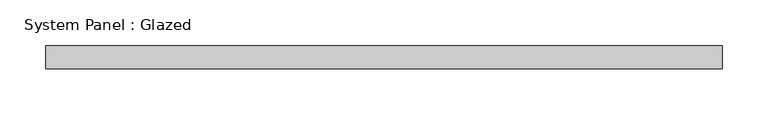
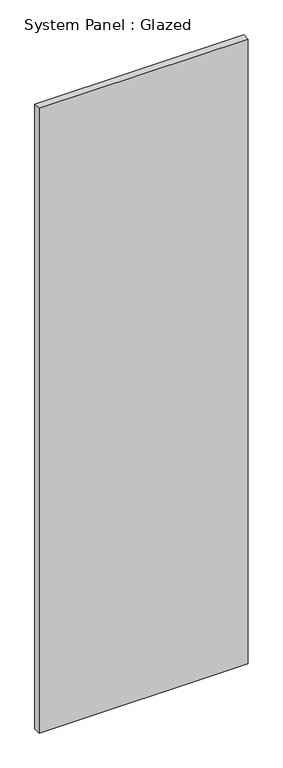
"""IFC4 building model written with IfcOpenShell, lengths in millimetres: plate geometry, System Panel : Glazed."""

from ifc_helpers import new_model, si_unit, origin, origin_with_axes, place, context, project, spatial, polyline, outline, extrude, source, transform, mapped, element, save


def system_panel_glazed_0d615b27(model_context):
    return source(origin(), model_context, "Body", "SweptSolid", [
        extrude(outline(polyline([(371.475, -44.45), (-371.475, -44.45), (-371.475, -19.05), (371.475, -19.05), (371.475, -44.45)])), origin_with_axes(), (0.0, 0.0, 1.0), 2343.15),
    ])


if __name__ == "__main__":
    model = new_model("IFC4")
    model_context = context("Model", 3, world=origin())
    ifc_project = project(units=[si_unit("LENGTHUNIT", "METRE", prefix="MILLI")], contexts=[model_context])
    site = spatial("IfcSite", under=ifc_project)
    building = spatial("IfcBuilding", under=site)
    placement = place(None, origin())
    system_panel_glazed_shape = system_panel_glazed_0d615b27(model_context)
    element("IfcPlate", 1, ObjectType="System Panel : Glazed", at=placement, inside=building, context=model_context, shape_type="MappedRepresentation", body=[
        mapped(system_panel_glazed_shape, transform((0.0, 0.0, 0.0), x_axis=(1.0, 0.0, 0.0), y_axis=(0.0, 1.0, 0.0), z_axis=(0.0, 0.0, 1.0))),
    ])
    save(model, "model.ifc")

# Revit data of these elements
# Type "System Panel : Glazed"
#   Construction Type Id = "GSP4R"
#   Analytic Construction = "1/8 in Pilkington single glazing"
#   Visual Light Transmittance = 0.9
#   Solar Heat Gain Coefficient = 0.86
#   Heat Transfer Coefficient (U) = 1.18115 BTU/(h·ft²·°F)
#   Define Thermal Properties by = 1
# Element 1 (IfcPlate, "System Panel : Glazed")
#   Materials on its faces: "glass panel 223"
# Materials
#   "glass panel 223": class "Generic", colour RGB 120 120 120, transparency 0, Cost = 0
